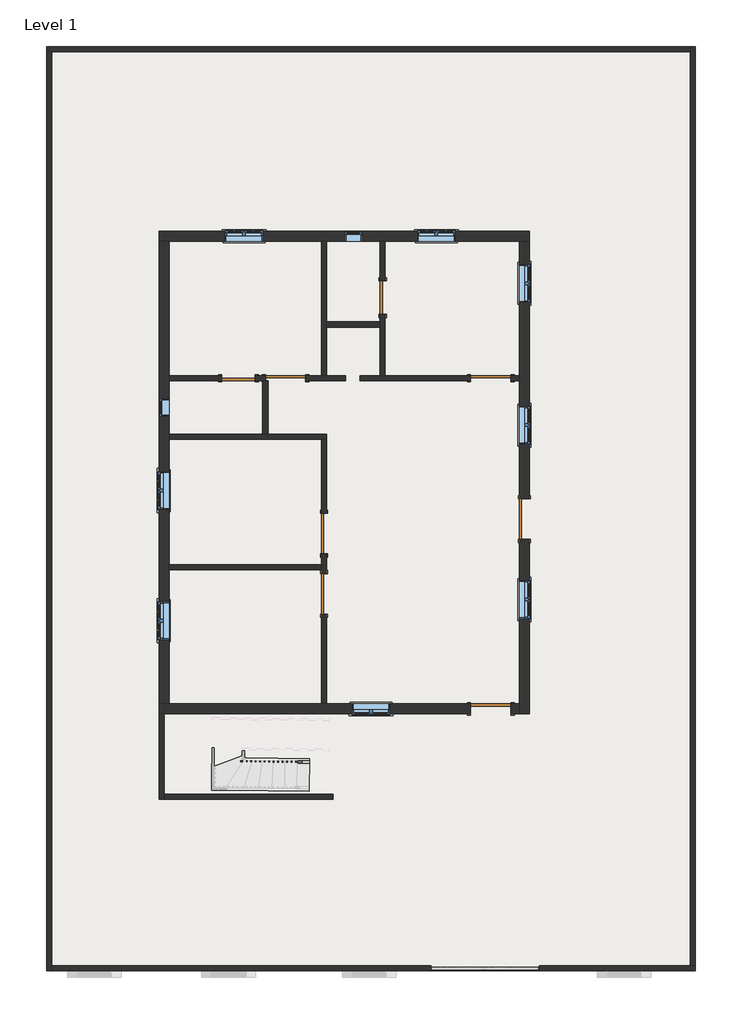
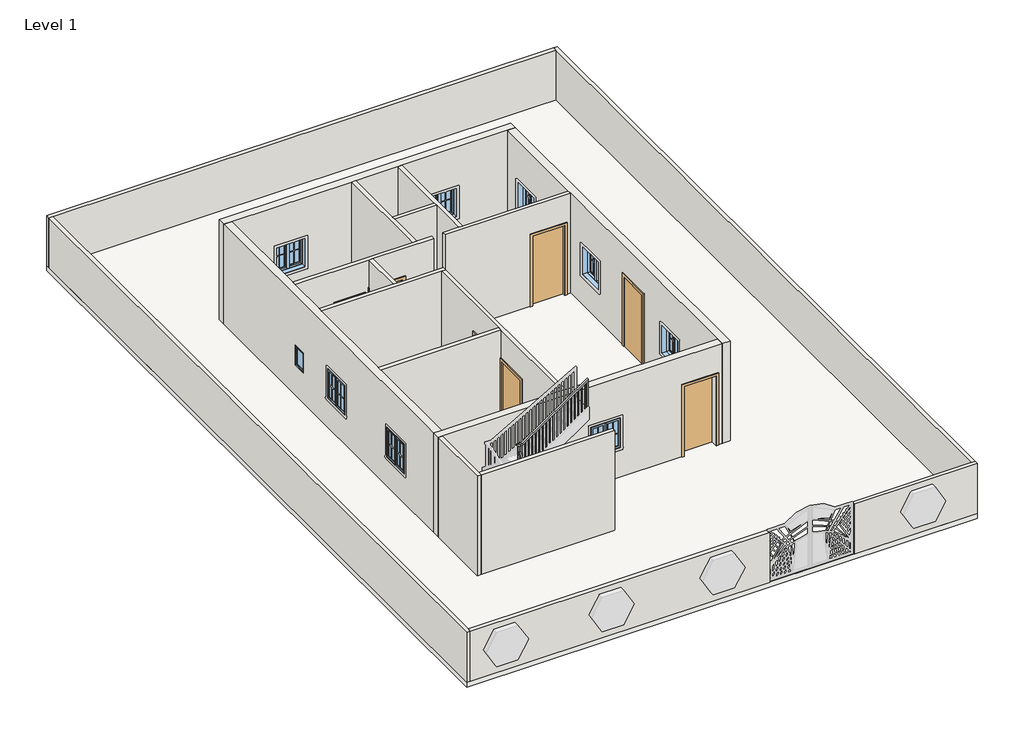
# One storey, part 1 of 2: 20 walls, 10 windows, 8 doors, 1 railing, 1 slab.
"""IFC4 building model written with IfcOpenShell, lengths in millimetres."""

from ifc_helpers import new_model, si_unit, frame, origin, origin_with_axes, place, context, project, spatial, polyline, outline, extrude, faceted_brep, transform, mapped, element, save
from components import door_f2b275c1, door_e5f9f3c4, door_305aa2a5, door_a90ba1ad, door_0ca8825f, window_aa618e30, window_339605e1

model = new_model("IFC4")

# Units and contexts
model_context = context("Model", 3, world=origin())
ifc_project = project(units=[si_unit("LENGTHUNIT", "METRE", prefix="MILLI")], contexts=[model_context])

# Site, building, storey
site = spatial("IfcSite", under=ifc_project)
building = spatial("IfcBuilding", under=site)
storey = spatial("IfcBuildingStorey", under=building, Name="Level 1", Elevation=0.0)

# Doors
placement = place(None, origin())
door_shape = door_f2b275c1(model_context)
element("IfcDoor", 1, ObjectType="Single-Flush : 30\" x 80\"", at=placement, inside=storey, context=model_context, shape_type="MappedRepresentation", body=[
    mapped(door_shape, transform((-295.4747832, 5557.2532079, 0.0), x_axis=(0.0, -1.0, 0.0), y_axis=(1.0, 0.0, 0.0), z_axis=(0.0, 0.0, 1.0))),
])
element("IfcDoor", 2, ObjectType="Single-Flush : 30\" x 80\"", at=placement, inside=storey, context=model_context, shape_type="MappedRepresentation", body=[
    mapped(door_shape, transform((-3572.0747832, 3728.4532079, 0.0), x_axis=(1.0, 0.0, 0.0), y_axis=(0.0, 1.0, 0.0), z_axis=(0.0, 0.0, 1.0))),
])
door_2_shape = door_e5f9f3c4(model_context)
element("IfcDoor", 3, ObjectType="Single-Flush : 36\" x 84\"", at=placement, inside=storey, context=model_context, shape_type="MappedRepresentation", body=[
    mapped(door_2_shape, transform((-2505.2747832, 3728.4532079, 0.0), x_axis=(1.0, 0.0, 0.0), y_axis=(0.0, 1.0, 0.0), z_axis=(0.0, 0.0, 1.0))),
])
element("IfcDoor", 4, ObjectType="Single-Flush : 36\" x 84\"", at=placement, inside=storey, context=model_context, shape_type="MappedRepresentation", body=[
    mapped(door_2_shape, transform((2161.9752168, 3728.4532079, 0.0), x_axis=(1.0, 0.0, 0.0), y_axis=(0.0, 1.0, 0.0), z_axis=(0.0, 0.0, 1.0))),
])
element("IfcDoor", 5, ObjectType="Single-Flush : 36\" x 84\"", at=placement, inside=storey, context=model_context, shape_type="MappedRepresentation", body=[
    mapped(door_2_shape, transform((-1628.9747832, -1173.7467921, 0.0), x_axis=(0.0, 1.0, 0.0), y_axis=(-1.0, 0.0, 0.0), z_axis=(0.0, 0.0, 1.0))),
])
door_3_shape = door_305aa2a5(model_context)
element("IfcDoor", 6, ObjectType="Single-Flush : 36\" x 84\"", at=placement, inside=storey, context=model_context, shape_type="MappedRepresentation", body=[
    mapped(door_3_shape, transform((-1628.9747832, 197.8532079, 0.0), x_axis=(0.0, -1.0, 0.0), y_axis=(1.0, 0.0, 0.0), z_axis=(0.0, 0.0, 1.0))),
])
door_4_shape = door_a90ba1ad(model_context)
element("IfcDoor", 7, ObjectType="Single-Flush : 36\" x 84\"", at=placement, inside=storey, context=model_context, shape_type="MappedRepresentation", body=[
    mapped(door_4_shape, transform((2923.9752168, 528.0532079, 0.0), x_axis=(0.0, -1.0, 0.0), y_axis=(1.0, 0.0, 0.0), z_axis=(0.0, 0.0, 1.0))),
])
door_5_shape = door_0ca8825f(model_context)
element("IfcDoor", 8, ObjectType="Single-Flush : 36\" x 84\"", at=placement, inside=storey, context=model_context, shape_type="MappedRepresentation", body=[
    mapped(door_5_shape, transform((2161.9752168, -3783.5967921, 0.0), x_axis=(1.0, 0.0, 0.0), y_axis=(0.0, 1.0, 0.0), z_axis=(0.0, 0.0, 1.0))),
])

# Railing
element("IfcRailing", 9, ObjectType="Handrail - Rectangular", at=placement, inside=storey, context=model_context, shape_type="SolidModel", body=[
    faceted_brep([(-1962.1803506, -5016.2038017, 1083.7333333), (-1962.1803506, -5016.2038017, 1022.2793596), (-1961.6349602, -4965.4067295, 1022.2793596), (-1961.6349602, -4965.4067295, 1083.7333333), (-3413.6283866, -5000.6201116, 2071.8756169), (-3464.4254588, -5000.0747212, 2045.0041661), (-3463.8800684, -4949.2776489, 2045.0041661), (-3413.0829962, -4949.8230393, 2071.8756169), (-3413.6283866, -5000.6201116, 2288.961538), (-3464.4254588, -5000.0747212, 2238.161538), (-3463.8800684, -4949.2776489, 2238.161538), (-3413.0829962, -4949.8230393, 2288.961538), (-3540.6210672, -4999.2566356, 2288.961538), (-3540.6210672, -4999.2566356, 2238.161538), (-3489.2786045, -4949.0049537, 2238.161538), (-3489.2786045, -4949.0049537, 2288.961538), (-3539.2575912, -4872.2639549, 2288.961538), (-3538.9677931, -4845.272478, 2238.161538), (-3488.1707209, -4845.8178684, 2238.161538), (-3488.4605189, -4872.8093453, 2288.961538), (-3537.8941152, -4745.2712743, 2477.0249579), (-3537.3487248, -4694.4742021, 2461.4786564), (-3486.5516525, -4695.0195925, 2461.4786564), (-3487.0970429, -4745.8166647, 2477.0249579), (-3537.8941152, -4745.2712743, 2645.076961), (-3537.3487248, -4694.4742021, 2594.276961), (-3486.5516525, -4695.0195925, 2594.276961), (-3487.0970429, -4745.8166647, 2645.076961), (-3536.5306392, -4618.2785937, 2645.076961), (-3536.5306392, -4618.2785937, 2594.276961), (-3486.2789573, -4669.6210563, 2594.276961), (-3486.2789573, -4669.6210563, 2645.076961), (-3409.5379585, -4619.6420697, 2645.076961), (-3393.6525863, -4619.8126254, 2594.276961), (-3394.1979767, -4670.6096976, 2594.276961), (-3410.0833489, -4670.439142, 2645.076961), (-1509.4062983, -4640.0431191, 3962.4), (-1509.9516887, -4690.8401913, 3962.4), (-1509.9516887, -4690.8401913, 3900.5869912), (-1509.4062983, -4640.0431191, 3900.5869912)], [[[0, 1, 2, 3]], [[1, 0, 4, 5]], [[2, 1, 5, 6]], [[3, 2, 6, 7]], [[0, 3, 7, 4]], [[5, 4, 8, 9]], [[6, 5, 9, 10]], [[7, 6, 10, 11]], [[4, 7, 11, 8]], [[9, 8, 12, 13]], [[10, 9, 13, 14]], [[11, 10, 14, 15]], [[8, 11, 15, 12]], [[13, 12, 16, 17]], [[14, 13, 17, 18]], [[15, 14, 18, 19]], [[12, 15, 19, 16]], [[17, 16, 20, 21]], [[18, 17, 21, 22]], [[19, 18, 22, 23]], [[16, 19, 23, 20]], [[21, 20, 24, 25]], [[22, 21, 25, 26]], [[23, 22, 26, 27]], [[20, 23, 27, 24]], [[25, 24, 28, 29]], [[26, 25, 29, 30]], [[27, 26, 30, 31]], [[24, 27, 31, 28]], [[29, 28, 32, 33]], [[30, 29, 33, 34]], [[31, 30, 34, 35]], [[28, 31, 35, 32]], [[36, 37, 38, 39]], [[33, 32, 36, 39]], [[34, 33, 39, 38]], [[35, 34, 38, 37]], [[32, 35, 37, 36]]]),
    extrude(outline(polyline([(221.9968897, -19.05), (235.2031102, 0.0), (1200.994449, 0.0), (1200.994449, -19.05), (221.9968897, -19.05)])), frame((-1590.7427644, -4674.0968508, 4079.6611157), z_axis=(0.01073603161956521, 0.9999423671517594, 0.0), x_axis=(0.0, 0.0, -1.0)), (0.0, 0.0, 1.0), 19.05),
    extrude(outline(polyline([(221.9968898, -19.05), (235.2031102, 0.0), (1130.5612733, 0.0), (1130.5612733, -19.05), (221.9968898, -19.05)])), frame((-1692.3369089, -4673.00607, 4009.22794), z_axis=(0.01073603161956521, 0.9999423671517594, 0.0), x_axis=(0.0, 0.0, -1.0)), (0.0, 0.0, 1.0), 19.05),
    extrude(outline(polyline([(221.9968897, -19.05), (235.2031102, 0.0), (1060.1280975, 0.0), (1060.1280975, -19.05), (221.9968897, -19.05)])), frame((-1793.9310534, -4671.9152892, 3938.7947642), z_axis=(0.01073603161956521, 0.9999423671517594, 0.0), x_axis=(0.0, 0.0, -1.0)), (0.0, 0.0, 1.0), 19.05),
    extrude(outline(polyline([(221.9968898, -19.05), (235.2031103, 0.0), (1159.0282552, 0.0), (1159.0282552, -19.05), (221.9968898, -19.05)])), frame((-1895.5251979, -4670.8245084, 3868.3615885), z_axis=(0.01073603161956521, 0.9999423671517594, 0.0), x_axis=(0.0, 0.0, -1.0)), (0.0, 0.0, 1.0), 19.05),
    extrude(outline(polyline([(221.9968898, -19.05), (235.2031102, 0.0), (1088.5950794, 0.0), (1088.5950794, -19.05), (221.9968898, -19.05)])), frame((-1997.1193424, -4669.7337275, 3797.9284127), z_axis=(0.01073603161956521, 0.9999423671517594, 0.0), x_axis=(0.0, 0.0, -1.0)), (0.0, 0.0, 1.0), 19.05),
    extrude(outline(polyline([(221.9968898, -19.05), (235.2031103, 0.0), (1187.495237, 0.0), (1187.495237, -19.05), (221.9968898, -19.05)])), frame((-2098.7134869, -4668.6429467, 3727.495237), z_axis=(0.01073603161956521, 0.9999423671517594, 0.0), x_axis=(0.0, 0.0, -1.0)), (0.0, 0.0, 1.0), 19.05),
    extrude(outline(polyline([(221.9968898, -19.05), (235.2031102, 0.0), (1117.0620612, 0.0), (1117.0620612, -19.05), (221.9968898, -19.05)])), frame((-2200.3076314, -4667.5521659, 3657.0620612), z_axis=(0.01073603161956521, 0.9999423671517594, 0.0), x_axis=(0.0, 0.0, -1.0)), (0.0, 0.0, 1.0), 19.05),
    extrude(outline(polyline([(221.9968897, -19.0499999), (235.2031102, 0.0), (1046.6288854, 0.0), (1046.6288854, -19.0499999), (221.9968897, -19.0499999)])), frame((-2301.9017759, -4666.4613851, 3586.6288854), z_axis=(0.01073603161956521, 0.9999423671517594, 0.0), x_axis=(0.0, 0.0, -1.0)), (0.0, 0.0, 1.0), 19.05),
    extrude(outline(polyline([(221.9968898, -19.0499999), (235.2031102, 0.0), (1145.529043, 0.0), (1145.529043, -19.0499999), (221.9968898, -19.0499999)])), frame((-2403.4959204, -4665.3706043, 3516.1957097), z_axis=(0.01073603161956521, 0.9999423671517594, 0.0), x_axis=(0.0, 0.0, -1.0)), (0.0, 0.0, 1.0), 19.05),
    extrude(outline(polyline([(221.9968897, -19.05), (235.2031102, 0.0), (1075.0958672, 0.0), (1075.0958672, -19.05), (221.9968897, -19.05)])), frame((-2505.090065, -4664.2798235, 3445.7625339), z_axis=(0.01073603161956521, 0.9999423671517594, 0.0), x_axis=(0.0, 0.0, -1.0)), (0.0, 0.0, 1.0), 19.05),
    extrude(outline(polyline([(221.9968898, -19.05), (235.2031103, 0.0), (1004.6626915, 0.0), (1004.6626915, -19.05), (221.9968898, -19.05)])), frame((-2606.6842095, -4663.1890427, 3375.3293582), z_axis=(0.01073603161956521, 0.9999423671517594, 0.0), x_axis=(0.0, 0.0, -1.0)), (0.0, 0.0, 1.0), 19.05),
    extrude(outline(polyline([(221.9968898, -19.05), (235.2031102, 0.0), (1103.5628491, 0.0), (1103.5628491, -19.05), (221.9968898, -19.05)])), frame((-2708.278354, -4662.0982619, 3304.8961824), z_axis=(0.01073603161956521, 0.9999423671517594, 0.0), x_axis=(0.0, 0.0, -1.0)), (0.0, 0.0, 1.0), 19.05),
    extrude(outline(polyline([(221.9968898, -19.05), (235.2031103, 0.0), (1033.1296734, 0.0), (1033.1296734, -19.05), (221.9968898, -19.05)])), frame((-2809.8724985, -4661.007481, 3234.4630067), z_axis=(0.01073603161956521, 0.9999423671517594, 0.0), x_axis=(0.0, 0.0, -1.0)), (0.0, 0.0, 1.0), 19.05),
    extrude(outline(polyline([(221.9968898, -19.05), (235.2031102, 0.0), (1132.0298309, 0.0), (1132.0298309, -19.05), (221.9968898, -19.05)])), frame((-2911.466643, -4659.9167002, 3164.0298309), z_axis=(0.01073603161956521, 0.9999423671517594, 0.0), x_axis=(0.0, 0.0, -1.0)), (0.0, 0.0, 1.0), 19.05),
    extrude(outline(polyline([(221.9968897, -19.05), (235.2031102, 0.0), (1061.5966551, 0.0), (1061.5966551, -19.05), (221.9968897, -19.05)])), frame((-3013.0607875, -4658.8259194, 3093.5966551), z_axis=(0.01073603161956521, 0.9999423671517594, 0.0), x_axis=(0.0, 0.0, -1.0)), (0.0, 0.0, 1.0), 19.05),
    extrude(outline(polyline([(221.9968898, -19.05), (235.2031102, 0.0), (991.1634794, 0.0), (991.1634794, -19.05), (221.9968898, -19.05)])), frame((-3114.654932, -4657.7351386, 3023.1634794), z_axis=(0.01073603161956521, 0.9999423671517594, 0.0), x_axis=(0.0, 0.0, -1.0)), (0.0, 0.0, 1.0), 19.05),
    extrude(outline(polyline([(221.9968897, -19.05), (235.2031102, 0.0), (1090.0636369, 0.0), (1090.0636369, -19.05), (221.9968897, -19.05)])), frame((-3216.2490765, -4656.6443578, 2952.7303036), z_axis=(0.01073603161956521, 0.9999423671517594, 0.0), x_axis=(0.0, 0.0, -1.0)), (0.0, 0.0, 1.0), 19.05),
    extrude(outline(polyline([(221.9968898, -19.05), (235.2031103, 0.0), (1019.6304612, 0.0), (1019.6304612, -19.05), (221.9968898, -19.05)])), frame((-3317.843221, -4655.553577, 2882.2971279), z_axis=(0.01073603161956521, 0.9999423671517594, 0.0), x_axis=(0.0, 0.0, -1.0)), (0.0, 0.0, 1.0), 19.05),
    extrude(outline(polyline([(221.9968898, -19.05), (235.2031102, 0.0), (1118.5306188, 0.0), (1118.5306188, -19.05), (221.9968898, -19.05)])), frame((-3419.4373655, -4654.4627962, 2811.8639521), z_axis=(0.01073603161956521, 0.9999423671517594, 0.0), x_axis=(0.0, 0.0, -1.0)), (0.0, 0.0, 1.0), 19.05),
    extrude(outline(polyline([(-3502.2553031, -4678.9750729), (-3521.3042052, -4678.7705515), (-3521.0996838, -4659.7216494), (-3502.0507817, -4659.9261708), (-3502.2553031, -4678.9750729)])), frame((0.0, 0.0, 1524.0), z_axis=(0.0, 0.0, 1.0), x_axis=(1.0, 0.0, 0.0)), (0.0, 0.0, 1.0), 1070.276961),
    extrude(outline(polyline([(214.4952435, -19.05), (242.7047565, 0.0), (1222.5739377, 0.0), (1222.5739377, -19.05), (214.4952435, -19.05)])), frame((-3503.3460839, -4780.5692174, 2577.2406044), z_axis=(-0.9999423671517594, 0.010736031619565895, 0.0), x_axis=(0.0, 0.0, -1.0)), (0.0, 0.0, 1.0), 19.05),
    extrude(outline(polyline([(214.4952435, -19.05), (242.7047565, 0.0), (1072.1232018, 0.0), (1072.1232018, -19.05), (214.4952435, -19.05)])), frame((-3504.4368647, -4882.1633619, 2426.7898685), z_axis=(-0.9999423671517594, 0.010736031619565895, 0.0), x_axis=(0.0, 0.0, -1.0)), (0.0, 0.0, 1.0), 19.05),
    extrude(outline(polyline([(-3476.1931112, -4965.0213631), (-3476.3976326, -4984.0702652), (-3495.4465347, -4983.8657438), (-3495.2420133, -4964.8168417), (-3476.1931112, -4965.0213631)])), frame((0.0, 0.0, 1185.3333333), z_axis=(0.0, 0.0, 1.0), x_axis=(1.0, 0.0, 0.0)), (0.0, 0.0, 1.0), 1052.8282047),
    extrude(outline(polyline([(235.0842231, -19.05), (222.115777, 0.0), (1203.1900014, 0.0), (1203.1900014, -19.05), (235.0842231, -19.05)])), frame((-3393.8523902, -4984.9565246, 2219.1900014), z_axis=(0.01073603161956537, 0.9999423671517593, 0.0), x_axis=(0.0, 0.0, -1.0)), (0.0, 0.0, 1.0), 19.05),
    extrude(outline(polyline([(235.084223, -19.05), (222.1157769, 0.0), (1134.0249555, 0.0), (1134.0249555, -19.05), (235.084223, -19.05)])), frame((-3292.2582457, -4986.0473054, 2150.0249555), z_axis=(0.01073603161956537, 0.9999423671517593, 0.0), x_axis=(0.0, 0.0, -1.0)), (0.0, 0.0, 1.0), 19.05),
    extrude(outline(polyline([(235.0842231, -19.05), (222.115777, 0.0), (1234.193243, 0.0), (1234.193243, -19.05), (235.0842231, -19.05)])), frame((-3190.6641012, -4987.1380862, 2080.8599097), z_axis=(0.01073603161956537, 0.9999423671517593, 0.0), x_axis=(0.0, 0.0, -1.0)), (0.0, 0.0, 1.0), 19.05),
    extrude(outline(polyline([(235.084223, -19.05), (222.1157769, 0.0), (1165.0281971, 0.0), (1165.0281971, -19.05), (235.084223, -19.05)])), frame((-3089.0699567, -4988.228867, 2011.6948638), z_axis=(0.01073603161956537, 0.9999423671517593, 0.0), x_axis=(0.0, 0.0, -1.0)), (0.0, 0.0, 1.0), 19.05),
    extrude(outline(polyline([(235.084223, -19.05), (222.1157769, 0.0), (1265.1964847, 0.0), (1265.1964847, -19.05), (235.084223, -19.05)])), frame((-2987.4758122, -4989.3196478, 1942.529818), z_axis=(0.01073603161956537, 0.9999423671517593, 0.0), x_axis=(0.0, 0.0, -1.0)), (0.0, 0.0, 1.0), 19.05),
    extrude(outline(polyline([(235.0842231, -19.05), (222.115777, 0.0), (1196.0314389, 0.0), (1196.0314389, -19.05), (235.0842231, -19.05)])), frame((-2885.8816677, -4990.4104286, 1873.3647722), z_axis=(0.01073603161956537, 0.9999423671517593, 0.0), x_axis=(0.0, 0.0, -1.0)), (0.0, 0.0, 1.0), 19.05),
    extrude(outline(polyline([(235.084223, -19.05), (222.1157769, 0.0), (1296.1997263, 0.0), (1296.1997263, -19.05), (235.084223, -19.05)])), frame((-2784.2875232, -4991.5012094, 1804.1997263), z_axis=(0.01073603161956537, 0.9999423671517593, 0.0), x_axis=(0.0, 0.0, -1.0)), (0.0, 0.0, 1.0), 19.05),
    extrude(outline(polyline([(235.0842231, -19.05), (222.115777, 0.0), (1227.0346805, 0.0), (1227.0346805, -19.05), (235.0842231, -19.05)])), frame((-2682.6933787, -4992.5919903, 1735.0346805), z_axis=(0.01073603161956537, 0.9999423671517593, 0.0), x_axis=(0.0, 0.0, -1.0)), (0.0, 0.0, 1.0), 19.05),
    extrude(outline(polyline([(235.084223, -19.05), (222.1157769, 0.0), (1157.8696346, 0.0), (1157.8696346, -19.05), (235.084223, -19.05)])), frame((-2581.0992342, -4993.6827711, 1665.8696346), z_axis=(0.01073603161956537, 0.9999423671517593, 0.0), x_axis=(0.0, 0.0, -1.0)), (0.0, 0.0, 1.0), 19.05),
    extrude(outline(polyline([(235.0842231, -19.05), (222.115777, 0.0), (1258.0379221, 0.0), (1258.0379221, -19.05), (235.0842231, -19.05)])), frame((-2479.5050897, -4994.7735519, 1596.7045888), z_axis=(0.01073603161956537, 0.9999423671517593, 0.0), x_axis=(0.0, 0.0, -1.0)), (0.0, 0.0, 1.0), 19.05),
    extrude(outline(polyline([(235.084223, -19.05), (222.1157769, 0.0), (1188.8728762, 0.0), (1188.8728762, -19.05), (235.084223, -19.05)])), frame((-2377.9109452, -4995.8643327, 1527.5395429), z_axis=(0.01073603161956537, 0.9999423671517593, 0.0), x_axis=(0.0, 0.0, -1.0)), (0.0, 0.0, 1.0), 19.05),
    extrude(outline(polyline([(235.084223, -19.05), (222.115777, 0.0), (1119.7078304, 0.0), (1119.7078304, -19.05), (235.084223, -19.05)])), frame((-2276.3168007, -4996.9551135, 1458.3744971), z_axis=(0.01073603161956537, 0.9999423671517593, 0.0), x_axis=(0.0, 0.0, -1.0)), (0.0, 0.0, 1.0), 19.05),
    extrude(outline(polyline([(235.0842231, -19.05), (222.115777, 0.0), (1219.876118, 0.0), (1219.876118, -19.05), (235.0842231, -19.05)])), frame((-2174.7226562, -4998.0458943, 1389.2094513), z_axis=(0.01073603161956537, 0.9999423671517593, 0.0), x_axis=(0.0, 0.0, -1.0)), (0.0, 0.0, 1.0), 19.05),
    extrude(outline(polyline([(235.084223, -19.05), (222.1157769, 0.0), (1150.7110721, 0.0), (1150.7110721, -19.05), (235.084223, -19.05)])), frame((-2073.1285117, -4999.1366751, 1320.0444054), z_axis=(0.01073603161956537, 0.9999423671517593, 0.0), x_axis=(0.0, 0.0, -1.0)), (0.0, 0.0, 1.0), 19.05),
    extrude(outline(polyline([(-3501.9826079, -4653.5765368), (-3521.03151, -4653.3720154), (-3520.8269886, -4634.3231133), (-3501.7780865, -4634.5276347), (-3501.9826079, -4653.5765368)])), frame((0.0, 0.0, 1524.0), z_axis=(0.0, 0.0, 1.0), x_axis=(1.0, 0.0, 0.0)), (0.0, 0.0, 1.0), 1070.276961),
    extrude(outline(polyline([(-3505.3231241, -4964.7086043), (-3505.5276455, -4983.7575064), (-3524.5765476, -4983.552985), (-3524.3720262, -4964.5040829), (-3505.3231241, -4964.7086043)])), frame((0.0, 0.0, 1185.3333333), z_axis=(0.0, 0.0, 1.0), x_axis=(1.0, 0.0, 0.0)), (0.0, 0.0, 1.0), 1052.8282047),
    extrude(outline(polyline([(221.9968897, -19.05), (235.2031102, 0.0), (1243.9172142, 0.0), (1243.9172142, -19.05), (221.9968897, -19.05)])), frame((-1528.8301563, -4674.7615848, 4122.5838809), z_axis=(0.01073603161956521, 0.9999423671517594, 0.0), x_axis=(0.0, 0.0, -1.0)), (0.0, 0.0, 1.0), 19.05),
    extrude(outline(polyline([(235.084223, -19.05), (222.1157769, 0.0), (1088.0302493, 0.0), (1088.0302493, -19.05), (235.084223, -19.05)])), frame((-1981.0588182, -5000.1251952, 1257.3635826), z_axis=(0.01073603161956537, 0.9999423671517593, 0.0), x_axis=(0.0, 0.0, -1.0)), (0.0, 0.0, 1.0), 19.05),
])

# Slab
element("IfcSlab", 10, ObjectType="Generic - 12\"", at=placement, inside=storey, context=model_context, shape_type="SweptSolid", body=[
    extrude(outline(polyline([(6808.4593371, 11261.08634), (6808.4593371, -9732.01366), (-7936.2406629, -9732.01366), (-7936.2406629, 11261.08634), (6808.4593371, 11261.08634)])), frame((0.0, 0.0, -152.4), z_axis=(0.0, 0.0, 1.0), x_axis=(1.0, 0.0, 0.0)), (0.0, 0.0, 1.0), 152.4),
])

# Walls
element("IfcWall", 11, ObjectType="WALL4.5\"", at=placement, inside=storey, context=model_context, shape_type="Brep", body=[
    faceted_brep([(-2048.0747832, 3671.3032079, 2133.6), (-2048.0747832, 3671.3032079, 0.0), (-1141.0287494, 3671.3032079, 0.0), (-1141.0287494, 3671.3032079, 3048.0), (-2905.3247832, 3671.3032079, 3048.0), (-3019.6247832, 3671.3032079, 3048.0), (-5153.2247832, 3671.3032079, 3048.0), (-5153.2247832, 3671.3032079, 0.0), (-3953.0747832, 3671.3032079, 0.0), (-3953.0747832, 3671.3032079, 2032.0), (-3191.0747832, 3671.3032079, 2032.0), (-3191.0747832, 3671.3032079, 0.0), (-3019.6247832, 3671.3032079, 0.0), (-2962.4747832, 3671.3032079, 0.0), (-2962.4747832, 3671.3032079, 2133.6), (-1141.0287494, 3785.6032079, 0.0), (-1571.8247832, 3785.6032079, 0.0), (-1686.1247832, 3785.6032079, 0.0), (-2048.0747832, 3785.6032079, 0.0), (-2048.0747832, 3785.6032079, 2133.6), (-2962.4747832, 3785.6032079, 2133.6), (-2962.4747832, 3785.6032079, 0.0), (-3191.0747832, 3785.6032079, 0.0), (-3191.0747832, 3785.6032079, 2032.0), (-3953.0747832, 3785.6032079, 2032.0), (-3953.0747832, 3785.6032079, 0.0), (-5153.2247832, 3785.6032079, 0.0), (-5153.2247832, 3785.6032079, 3048.0), (-1686.1247832, 3785.6032079, 3048.0), (-1571.8247832, 3785.6032079, 3048.0), (-1141.0287494, 3785.6032079, 3048.0)], [[[0, 1, 2, 3, 4, 5, 6, 7, 8, 9, 10, 11, 12, 13, 14]], [[15, 16, 17, 18, 19, 20, 21, 22, 23, 24, 25, 26, 27, 28, 29, 30]], [[8, 7, 26, 25]], [[2, 1, 18, 17, 16, 15]], [[13, 12, 11, 22, 21]], [[3, 2, 15, 30]], [[7, 6, 27, 26]], [[23, 22, 11, 10]], [[24, 23, 10, 9]], [[25, 24, 9, 8]], [[19, 18, 1, 0]], [[20, 19, 0, 14]], [[21, 20, 14, 13]], [[6, 5, 4, 3, 30, 29, 28, 27]]]),
])
element("IfcWall", 12, ObjectType="WALL4.5\"", at=placement, inside=storey, context=model_context, shape_type="Brep", body=[
    faceted_brep([(2619.1752168, 3671.3032079, 2133.6), (2619.1752168, 3671.3032079, 0.0), (2809.6752168, 3671.3032079, 0.0), (2809.6752168, 3671.3032079, 3048.0), (-812.7163761, 3671.3032079, 3048.0), (-812.7163761, 3671.3032079, 0.0), (1704.7752168, 3671.3032079, 0.0), (1704.7752168, 3671.3032079, 2133.6), (2809.6752168, 3785.6032079, 0.0), (2619.1752168, 3785.6032079, 0.0), (2619.1752168, 3785.6032079, 2133.6), (1704.7752168, 3785.6032079, 2133.6), (1704.7752168, 3785.6032079, 0.0), (-238.3247832, 3785.6032079, 0.0), (-352.6247832, 3785.6032079, 0.0), (-812.7163761, 3785.6032079, 0.0), (-812.7163761, 3785.6032079, 3048.0), (-352.6247832, 3785.6032079, 3048.0), (-238.3247832, 3785.6032079, 3048.0), (2809.6752168, 3785.6032079, 3048.0)], [[[0, 1, 2, 3, 4, 5, 6, 7]], [[8, 9, 10, 11, 12, 13, 14, 15, 16, 17, 18, 19]], [[6, 5, 15, 14, 13, 12]], [[2, 1, 9, 8]], [[5, 4, 16, 15]], [[3, 2, 8, 19]], [[10, 9, 1, 0]], [[11, 10, 0, 7]], [[12, 11, 7, 6]], [[4, 3, 19, 18, 17, 16]]]),
])
element("IfcWall", 13, ObjectType="WALL4.5\"", at=placement, inside=storey, context=model_context, shape_type="Brep", body=[
    faceted_brep([(-1686.1247832, 6833.6032079, 0.0), (-1686.1247832, 3785.6032079, 0.0), (-1686.1247832, 3785.6032079, 3048.0), (-1686.1247832, 6833.6032079, 3048.0), (-1571.8247832, 6833.6032079, 0.0), (-1571.8247832, 6833.6032079, 3048.0), (-1571.8247832, 5004.8032079, 3048.0), (-1571.8247832, 4890.5032079, 3048.0), (-1571.8247832, 3785.6032079, 3048.0), (-1571.8247832, 3785.6032079, 0.0), (-1571.8247832, 4890.5032079, 0.0), (-1571.8247832, 5004.8032079, 0.0)], [[[0, 1, 2, 3]], [[4, 5, 6, 7, 8, 9, 10, 11]], [[1, 0, 4, 11, 10, 9]], [[0, 3, 5, 4]], [[2, 1, 9, 8]], [[3, 2, 8, 7, 6, 5]]]),
])
element("IfcWall", 14, ObjectType="WALL4.5\"", at=placement, inside=storey, context=model_context, shape_type="SweptSolid", body=[
    extrude(outline(polyline([(-352.6247832, 4890.5032079), (-1571.8247832, 4890.5032079), (-1571.8247832, 5004.8032079), (-352.6247832, 5004.8032079), (-352.6247832, 4890.5032079)])), origin_with_axes(), (0.0, 0.0, 1.0), 3048.0),
])
element("IfcWall", 15, ObjectType="WALL4.5\"", at=placement, inside=storey, context=model_context, shape_type="Brep", body=[
    faceted_brep([(-352.6247832, 5176.2532079, 2032.0), (-352.6247832, 5176.2532079, 0.0), (-352.6247832, 5004.8032079, 0.0), (-352.6247832, 4890.5032079, 0.0), (-352.6247832, 3785.6032079, 0.0), (-352.6247832, 3785.6032079, 3048.0), (-352.6247832, 4890.5032079, 3048.0), (-352.6247832, 5004.8032079, 3048.0), (-352.6247832, 6833.6032079, 3048.0), (-352.6247832, 6833.6032079, 0.0), (-352.6247832, 5938.2532079, 0.0), (-352.6247832, 5938.2532079, 2032.0), (-238.3247832, 3785.6032079, 0.0), (-238.3247832, 5176.2532079, 0.0), (-238.3247832, 5176.2532079, 2032.0), (-238.3247832, 5938.2532079, 2032.0), (-238.3247832, 5938.2532079, 0.0), (-238.3247832, 6833.6032079, 0.0), (-238.3247832, 6833.6032079, 3048.0), (-238.3247832, 3785.6032079, 3048.0)], [[[0, 1, 2, 3, 4, 5, 6, 7, 8, 9, 10, 11]], [[12, 13, 14, 15, 16, 17, 18, 19]], [[10, 9, 17, 16]], [[4, 3, 2, 1, 13, 12]], [[9, 8, 18, 17]], [[5, 4, 12, 19]], [[14, 13, 1, 0]], [[15, 14, 0, 11]], [[16, 15, 11, 10]], [[8, 7, 6, 5, 19, 18]]]),
])
element("IfcWall", 16, ObjectType="WALL4.5\"", at=placement, inside=storey, context=model_context, shape_type="Brep", body=[
    faceted_brep([(-3019.6247832, 3671.3032079, 0.0), (-3019.6247832, 2452.1032079, 0.0), (-3019.6247832, 2452.1032079, 3048.0), (-3019.6247832, 3671.3032079, 3048.0), (-2905.3247832, 3671.3032079, 0.0), (-2905.3247832, 3671.3032079, 3048.0), (-2905.3247832, 2452.1032079, 3048.0), (-2905.3247832, 2452.1032079, 0.0), (-2962.4747832, 3671.3032079, 0.0)], [[[0, 1, 2, 3]], [[4, 5, 6, 7]], [[1, 0, 8, 4, 7]], [[0, 3, 5, 4, 8]], [[2, 1, 7, 6]], [[3, 2, 6, 5]]]),
])
element("IfcWall", 17, ObjectType="WALL4.5\"", at=placement, inside=storey, context=model_context, shape_type="Brep", body=[
    faceted_brep([(-5153.2247832, 2337.8032079, 0.0), (-1686.1247832, 2337.8032079, 0.0), (-1571.8247832, 2337.8032079, 0.0), (-1571.8247832, 2337.8032079, 3048.0), (-1686.1247832, 2337.8032079, 3048.0), (-5153.2247832, 2337.8032079, 3048.0), (-5153.2247832, 2452.1032079, 0.0), (-5153.2247832, 2452.1032079, 3048.0), (-3019.6247832, 2452.1032079, 3048.0), (-2905.3247832, 2452.1032079, 3048.0), (-1571.8247832, 2452.1032079, 3048.0), (-1571.8247832, 2452.1032079, 0.0), (-2905.3247832, 2452.1032079, 0.0), (-3019.6247832, 2452.1032079, 0.0)], [[[0, 1, 2, 3, 4, 5]], [[6, 7, 8, 9, 10, 11, 12, 13]], [[2, 1, 0, 6, 13, 12, 11]], [[0, 5, 7, 6]], [[3, 2, 11, 10]], [[5, 4, 3, 10, 9, 8, 7]]]),
])
element("IfcWall", 18, ObjectType="WALL4.5\"", at=placement, inside=storey, context=model_context, shape_type="Brep", body=[
    faceted_brep([(-1686.1247832, -259.3467921, 0.0), (-1686.1247832, -506.9967921, 0.0), (-1686.1247832, -621.2967921, 0.0), (-1686.1247832, -716.5467921, 0.0), (-1686.1247832, -716.5467921, 2133.6), (-1686.1247832, -1630.9467921, 2133.6), (-1686.1247832, -1630.9467921, 0.0), (-1686.1247832, -3669.2967921, 0.0), (-1686.1247832, -3669.2967921, 3048.0), (-1686.1247832, -621.2967921, 3048.0), (-1686.1247832, -506.9967921, 3048.0), (-1686.1247832, 2337.8032079, 3048.0), (-1686.1247832, 2337.8032079, 0.0), (-1686.1247832, 655.0532079, 0.0), (-1686.1247832, 655.0532079, 2133.6), (-1686.1247832, -259.3467921, 2133.6), (-1571.8247832, -716.5467921, 2133.6), (-1571.8247832, -716.5467921, 0.0), (-1571.8247832, -259.3467921, 0.0), (-1571.8247832, -259.3467921, 2133.6), (-1571.8247832, 655.0532079, 2133.6), (-1571.8247832, 655.0532079, 0.0), (-1571.8247832, 2337.8032079, 0.0), (-1571.8247832, 2337.8032079, 3048.0), (-1571.8247832, -3669.2967921, 3048.0), (-1571.8247832, -3669.2967921, 0.0), (-1571.8247832, -1630.9467921, 0.0), (-1571.8247832, -1630.9467921, 2133.6)], [[[0, 1, 2, 3, 4, 5, 6, 7, 8, 9, 10, 11, 12, 13, 14, 15]], [[16, 17, 18, 19, 20, 21, 22, 23, 24, 25, 26, 27]], [[13, 12, 22, 21]], [[26, 25, 7, 6]], [[18, 17, 3, 2, 1, 0]], [[12, 11, 23, 22]], [[8, 7, 25, 24]], [[19, 18, 0, 15]], [[20, 19, 15, 14]], [[21, 20, 14, 13]], [[4, 3, 17, 16]], [[5, 4, 16, 27]], [[6, 5, 27, 26]], [[11, 10, 9, 8, 24, 23]]]),
])
element("IfcWall", 19, ObjectType="WALL4.5\"", at=placement, inside=storey, context=model_context, shape_type="SweptSolid", body=[
    extrude(outline(polyline([(-1686.1247832, -621.2967921), (-5153.2247832, -621.2967921), (-5153.2247832, -506.9967921), (-1686.1247832, -506.9967921), (-1686.1247832, -621.2967921)])), origin_with_axes(), (0.0, 0.0, 1.0), 3048.0),
])
element("IfcWall", 20, ObjectType="WALL4.5\"", at=placement, inside=storey, context=model_context, shape_type="Brep", body=[
    faceted_brep([(-5381.8247832, -3897.8967921, 0.0), (-5381.8247832, -5840.9967921, 0.0), (-5381.8247832, -5840.9967921, 3048.0), (-5381.8247832, -3897.8967921, 3048.0), (-5267.5247832, -3897.8967921, 0.0), (-5267.5247832, -3897.8967921, 3048.0), (-5267.5247832, -5726.6967921, 3048.0), (-5267.5247832, -5840.9967921, 3048.0), (-5267.5247832, -5840.9967921, 0.0), (-5267.5247832, -5726.6967921, 0.0)], [[[0, 1, 2, 3]], [[4, 5, 6, 7, 8, 9]], [[1, 0, 4, 9, 8]], [[0, 3, 5, 4]], [[2, 1, 8, 7]], [[3, 2, 7, 6, 5]]]),
])
element("IfcWall", 21, ObjectType="WALL4.5\"", at=placement, inside=storey, context=model_context, shape_type="SweptSolid", body=[
    extrude(outline(polyline([(-1419.4247832, -5840.9967921), (-5267.5247832, -5840.9967921), (-5267.5247832, -5726.6967921), (-1419.4247832, -5726.6967921), (-1419.4247832, -5840.9967921)])), origin_with_axes(), (0.0, 0.0, 1.0), 3048.0),
])
element("IfcWall", 22, ObjectType="WALL4.5\"", at=placement, inside=storey, context=model_context, shape_type="Brep", body=[
    faceted_brep([(-7936.2406629, 11146.78634, 0.0), (-7821.9406629, 11146.78634, 0.0), (6694.1593371, 11146.78634, 0.0), (6694.1593371, 11146.78634, 1524.0), (-7821.9406629, 11146.78634, 1524.0), (-7936.2406629, 11146.78634, 1524.0), (-7936.2406629, 11261.08634, 0.0), (-7936.2406629, 11261.08634, 1524.0), (6694.1593371, 11261.08634, 1524.0), (6694.1593371, 11261.08634, 0.0)], [[[0, 1, 2, 3, 4, 5]], [[6, 7, 8, 9]], [[2, 1, 0, 6, 9]], [[5, 4, 3, 8, 7]], [[0, 5, 7, 6]], [[3, 2, 9, 8]]]),
])
element("IfcWall", 23, ObjectType="WALL4.5\"", at=placement, inside=storey, context=model_context, shape_type="Brep", body=[
    faceted_brep([(-7821.9406629, -9732.01366, 0.0), (-7821.9406629, -9617.71366, 0.0), (-7821.9406629, 11146.78634, 0.0), (-7821.9406629, 11146.78634, 1524.0), (-7821.9406629, -9617.71366, 1524.0), (-7821.9406629, -9732.01366, 1524.0), (-7936.2406629, -9732.01366, 0.0), (-7936.2406629, -9732.01366, 1524.0), (-7936.2406629, 11146.78634, 1524.0), (-7936.2406629, 11146.78634, 0.0)], [[[0, 1, 2, 3, 4, 5]], [[6, 7, 8, 9]], [[2, 1, 0, 6, 9]], [[5, 4, 3, 8, 7]], [[0, 5, 7, 6]], [[3, 2, 9, 8]]]),
])
element("IfcWall", 24, ObjectType="WALL4.5\"", at=placement, inside=storey, context=model_context, shape_type="Brep", body=[
    faceted_brep([(6808.4593371, -9617.71366, 0.0), (6694.1593371, -9617.71366, 0.0), (3271.5093371, -9617.71366, 0.0), (3271.5093371, -9617.71366, 1524.0), (6694.1593371, -9617.71366, 1524.0), (6808.4593371, -9617.71366, 1524.0), (6808.4593371, -9732.01366, 0.0), (6808.4593371, -9732.01366, 1524.0), (3271.5093371, -9732.01366, 1524.0), (3271.5093371, -9732.01366, 0.0)], [[[0, 1, 2, 3, 4, 5]], [[6, 7, 8, 9]], [[2, 1, 0, 6, 9]], [[3, 2, 9, 8]], [[5, 4, 3, 8, 7]], [[0, 5, 7, 6]]]),
])
element("IfcWall", 25, ObjectType="WALL4.5\"", at=placement, inside=storey, context=model_context, shape_type="Brep", body=[
    faceted_brep([(6694.1593371, 11261.08634, 0.0), (6694.1593371, 11146.78634, 0.0), (6694.1593371, -9617.71366, 0.0), (6694.1593371, -9617.71366, 1524.0), (6694.1593371, 11146.78634, 1524.0), (6694.1593371, 11261.08634, 1524.0), (6808.4593371, 11261.08634, 0.0), (6808.4593371, 11261.08634, 1524.0), (6808.4593371, -9617.71366, 1524.0), (6808.4593371, -9617.71366, 0.0)], [[[0, 1, 2, 3, 4, 5]], [[6, 7, 8, 9]], [[2, 1, 0, 6, 9]], [[5, 4, 3, 8, 7]], [[0, 5, 7, 6]], [[3, 2, 9, 8]]]),
])
element("IfcWall", 26, ObjectType="WALL4.5\"", at=placement, inside=storey, context=model_context, shape_type="SweptSolid", body=[
    extrude(outline(polyline([(-7821.9406629, -9617.71366), (807.7093371, -9617.71366), (807.7093371, -9732.01366), (-7821.9406629, -9732.01366), (-7821.9406629, -9617.71366)])), origin_with_axes(), (0.0, 0.0, 1.0), 1524.0),
])
element("IfcWall", 27, ObjectType="WALL9\"", at=placement, inside=storey, context=model_context, shape_type="Brep", body=[
    faceted_brep([(-5381.8247832, 6833.6032079, 0.0), (-5153.2247832, 6833.6032079, 0.0), (-1686.1247832, 6833.6032079, 0.0), (-1571.8247832, 6833.6032079, 0.0), (-352.6247832, 6833.6032079, 0.0), (-238.3247832, 6833.6032079, 0.0), (2809.6752168, 6833.6032079, 0.0), (3038.2752168, 6833.6032079, 0.0), (3038.2752168, 6833.6032079, 3048.0), (2809.6752168, 6833.6032079, 3048.0), (-238.3247832, 6833.6032079, 3048.0), (-352.6247832, 6833.6032079, 3048.0), (-1571.8247832, 6833.6032079, 3048.0), (-1686.1247832, 6833.6032079, 3048.0), (-5153.2247832, 6833.6032079, 3048.0), (-5381.8247832, 6833.6032079, 3048.0), (-759.0247832, 6833.6032079, 1524.0), (-759.0247832, 6833.6032079, 914.4), (-1165.4247832, 6833.6032079, 914.4), (-1165.4247832, 6833.6032079, 1524.0), (-3016.4497832, 6833.6032079, 1828.8), (-3016.4497832, 6833.6032079, 914.4), (-3880.0497832, 6833.6032079, 914.4), (-3880.0497832, 6833.6032079, 1828.8), (1355.5252168, 6833.6032079, 1828.8), (1355.5252168, 6833.6032079, 914.4), (491.9252168, 6833.6032079, 914.4), (491.9252168, 6833.6032079, 1828.8), (-5381.8247832, 7062.2032079, 0.0), (-5381.8247832, 7062.2032079, 3048.0), (3038.2752168, 7062.2032079, 3048.0), (3038.2752168, 7062.2032079, 0.0), (-759.0247832, 7062.2032079, 1524.0), (-1165.4247832, 7062.2032079, 1524.0), (-1165.4247832, 7062.2032079, 914.4), (-759.0247832, 7062.2032079, 914.4), (-3016.4497832, 7062.2032079, 1828.8), (-3880.0497832, 7062.2032079, 1828.8), (-3880.0497832, 7062.2032079, 914.4), (-3016.4497832, 7062.2032079, 914.4), (1355.5252168, 7062.2032079, 1828.8), (491.9252168, 7062.2032079, 1828.8), (491.9252168, 7062.2032079, 914.4), (1355.5252168, 7062.2032079, 914.4)], [[[0, 1, 2, 3, 4, 5, 6, 7, 8, 9, 10, 11, 12, 13, 14, 15], [16, 17, 18, 19], [20, 21, 22, 23], [24, 25, 26, 27]], [[28, 29, 30, 31], [32, 33, 34, 35], [36, 37, 38, 39], [40, 41, 42, 43]], [[7, 6, 5, 4, 3, 2, 1, 0, 28, 31]], [[8, 7, 31, 30]], [[0, 15, 29, 28]], [[17, 16, 32, 35]], [[18, 17, 35, 34]], [[19, 18, 34, 33]], [[16, 19, 33, 32]], [[21, 20, 36, 39]], [[22, 21, 39, 38]], [[23, 22, 38, 37]], [[20, 23, 37, 36]], [[25, 24, 40, 43]], [[26, 25, 43, 42]], [[27, 26, 42, 41]], [[24, 27, 41, 40]], [[15, 14, 13, 12, 11, 10, 9, 8, 30, 29]]]),
])
element("IfcWall", 28, ObjectType="WALL9\"", at=placement, inside=storey, context=model_context, shape_type="Brep", body=[
    faceted_brep([(2809.6752168, 70.8532079, 2133.6), (2809.6752168, 70.8532079, 0.0), (2809.6752168, -3669.2967921, 0.0), (2809.6752168, -3897.8967921, 0.0), (2809.6752168, -3897.8967921, 3048.0), (2809.6752168, -3669.2967921, 3048.0), (2809.6752168, 3671.3032079, 3048.0), (2809.6752168, 3785.6032079, 3048.0), (2809.6752168, 6833.6032079, 3048.0), (2809.6752168, 6833.6032079, 0.0), (2809.6752168, 3785.6032079, 0.0), (2809.6752168, 3671.3032079, 0.0), (2809.6752168, 985.2532079, 0.0), (2809.6752168, 985.2532079, 2133.6), (2809.6752168, 5449.3032079, 1828.8), (2809.6752168, 5449.3032079, 914.4), (2809.6752168, 6312.9032079, 914.4), (2809.6752168, 6312.9032079, 1828.8), (2809.6752168, 2229.8532079, 1828.8), (2809.6752168, 2229.8532079, 914.4), (2809.6752168, 3093.4532079, 914.4), (2809.6752168, 3093.4532079, 1828.8), (2809.6752168, -1732.5467921, 1828.8), (2809.6752168, -1732.5467921, 914.4), (2809.6752168, -868.9467921, 914.4), (2809.6752168, -868.9467921, 1828.8), (3038.2752168, -3897.8967921, 0.0), (3038.2752168, 70.8532079, 0.0), (3038.2752168, 70.8532079, 2133.6), (3038.2752168, 985.2532079, 2133.6), (3038.2752168, 985.2532079, 0.0), (3038.2752168, 6833.6032079, 0.0), (3038.2752168, 6833.6032079, 3048.0), (3038.2752168, -3897.8967921, 3048.0), (3038.2752168, 5449.3032079, 1828.8), (3038.2752168, 6312.9032079, 1828.8), (3038.2752168, 6312.9032079, 914.4), (3038.2752168, 5449.3032079, 914.4), (3038.2752168, 2229.8532079, 1828.8), (3038.2752168, 3093.4532079, 1828.8), (3038.2752168, 3093.4532079, 914.4), (3038.2752168, 2229.8532079, 914.4), (3038.2752168, -1732.5467921, 1828.8), (3038.2752168, -868.9467921, 1828.8), (3038.2752168, -868.9467921, 914.4), (3038.2752168, -1732.5467921, 914.4)], [[[0, 1, 2, 3, 4, 5, 6, 7, 8, 9, 10, 11, 12, 13], [14, 15, 16, 17], [18, 19, 20, 21], [22, 23, 24, 25]], [[26, 27, 28, 29, 30, 31, 32, 33], [34, 35, 36, 37], [38, 39, 40, 41], [42, 43, 44, 45]], [[3, 2, 1, 27, 26]], [[12, 11, 10, 9, 31, 30]], [[9, 8, 32, 31]], [[4, 3, 26, 33]], [[28, 27, 1, 0]], [[29, 28, 0, 13]], [[30, 29, 13, 12]], [[15, 14, 34, 37]], [[16, 15, 37, 36]], [[17, 16, 36, 35]], [[14, 17, 35, 34]], [[19, 18, 38, 41]], [[20, 19, 41, 40]], [[21, 20, 40, 39]], [[18, 21, 39, 38]], [[23, 22, 42, 45]], [[24, 23, 45, 44]], [[25, 24, 44, 43]], [[22, 25, 43, 42]], [[8, 7, 6, 5, 4, 33, 32]]]),
])
element("IfcWall", 29, ObjectType="WALL9\"", at=placement, inside=storey, context=model_context, shape_type="Brep", body=[
    faceted_brep([(2809.6752168, -3669.2967921, 0.0), (2619.1752168, -3669.2967921, 0.0), (2619.1752168, -3669.2967921, 2133.6), (1704.7752168, -3669.2967921, 2133.6), (1704.7752168, -3669.2967921, 0.0), (-1571.8247832, -3669.2967921, 0.0), (-1686.1247832, -3669.2967921, 0.0), (-5153.2247832, -3669.2967921, 0.0), (-5381.8247832, -3669.2967921, 0.0), (-5381.8247832, -3669.2967921, 3048.0), (-5153.2247832, -3669.2967921, 3048.0), (-1686.1247832, -3669.2967921, 3048.0), (-1571.8247832, -3669.2967921, 3048.0), (2809.6752168, -3669.2967921, 3048.0), (-993.9747832, -3669.2967921, 1828.8), (-993.9747832, -3669.2967921, 914.4), (-130.3747832, -3669.2967921, 914.4), (-130.3747832, -3669.2967921, 1828.8), (2619.1752168, -3897.8967921, 2133.6), (2619.1752168, -3897.8967921, 0.0), (2809.6752168, -3897.8967921, 0.0), (2809.6752168, -3897.8967921, 3048.0), (-5267.5247832, -3897.8967921, 3048.0), (-5381.8247832, -3897.8967921, 3048.0), (-5381.8247832, -3897.8967921, 0.0), (-5267.5247832, -3897.8967921, 0.0), (1704.7752168, -3897.8967921, 0.0), (1704.7752168, -3897.8967921, 2133.6), (-993.9747832, -3897.8967921, 1828.8), (-130.3747832, -3897.8967921, 1828.8), (-130.3747832, -3897.8967921, 914.4), (-993.9747832, -3897.8967921, 914.4)], [[[0, 1, 2, 3, 4, 5, 6, 7, 8, 9, 10, 11, 12, 13], [14, 15, 16, 17]], [[18, 19, 20, 21, 22, 23, 24, 25, 26, 27], [28, 29, 30, 31]], [[20, 19, 1, 0]], [[26, 25, 24, 8, 7, 6, 5, 4]], [[0, 13, 21, 20]], [[9, 8, 24, 23]], [[2, 1, 19, 18]], [[3, 2, 18, 27]], [[4, 3, 27, 26]], [[15, 14, 28, 31]], [[16, 15, 31, 30]], [[17, 16, 30, 29]], [[14, 17, 29, 28]], [[13, 12, 11, 10, 9, 23, 22, 21]]]),
])
element("IfcWall", 30, ObjectType="WALL9\"", at=placement, inside=storey, context=model_context, shape_type="Brep", body=[
    faceted_brep([(-5153.2247832, -3669.2967921, 0.0), (-5153.2247832, -621.2967921, 0.0), (-5153.2247832, -506.9967921, 0.0), (-5153.2247832, 2337.8032079, 0.0), (-5153.2247832, 2452.1032079, 0.0), (-5153.2247832, 3671.3032079, 0.0), (-5153.2247832, 3785.6032079, 0.0), (-5153.2247832, 6833.6032079, 0.0), (-5153.2247832, 6833.6032079, 3048.0), (-5153.2247832, 3785.6032079, 3048.0), (-5153.2247832, 3671.3032079, 3048.0), (-5153.2247832, 2452.1032079, 3048.0), (-5153.2247832, 2337.8032079, 3048.0), (-5153.2247832, -506.9967921, 3048.0), (-5153.2247832, -621.2967921, 3048.0), (-5153.2247832, -3669.2967921, 3048.0), (-5153.2247832, 3264.9032079, 1524.0), (-5153.2247832, 3264.9032079, 914.4), (-5153.2247832, 2858.5032079, 914.4), (-5153.2247832, 2858.5032079, 1524.0), (-5153.2247832, 1607.5532079, 1828.8), (-5153.2247832, 1607.5532079, 914.4), (-5153.2247832, 743.9532079, 914.4), (-5153.2247832, 743.9532079, 1828.8), (-5153.2247832, -1351.5467921, 1828.8), (-5153.2247832, -1351.5467921, 914.4), (-5153.2247832, -2215.1467921, 914.4), (-5153.2247832, -2215.1467921, 1828.8), (-5381.8247832, -3669.2967921, 0.0), (-5381.8247832, -3669.2967921, 3048.0), (-5381.8247832, 6833.6032079, 3048.0), (-5381.8247832, 6833.6032079, 0.0), (-5381.8247832, 3264.9032079, 1524.0), (-5381.8247832, 2858.5032079, 1524.0), (-5381.8247832, 2858.5032079, 914.4), (-5381.8247832, 3264.9032079, 914.4), (-5381.8247832, 1607.5532079, 1828.8), (-5381.8247832, 743.9532079, 1828.8), (-5381.8247832, 743.9532079, 914.4), (-5381.8247832, 1607.5532079, 914.4), (-5381.8247832, -1351.5467921, 1828.8), (-5381.8247832, -2215.1467921, 1828.8), (-5381.8247832, -2215.1467921, 914.4), (-5381.8247832, -1351.5467921, 914.4)], [[[0, 1, 2, 3, 4, 5, 6, 7, 8, 9, 10, 11, 12, 13, 14, 15], [16, 17, 18, 19], [20, 21, 22, 23], [24, 25, 26, 27]], [[28, 29, 30, 31], [32, 33, 34, 35], [36, 37, 38, 39], [40, 41, 42, 43]], [[7, 6, 5, 4, 3, 2, 1, 0, 28, 31]], [[8, 7, 31, 30]], [[0, 15, 29, 28]], [[17, 16, 32, 35]], [[18, 17, 35, 34]], [[19, 18, 34, 33]], [[16, 19, 33, 32]], [[21, 20, 36, 39]], [[22, 21, 39, 38]], [[23, 22, 38, 37]], [[20, 23, 37, 36]], [[25, 24, 40, 43]], [[26, 25, 43, 42]], [[27, 26, 42, 41]], [[24, 27, 41, 40]], [[15, 14, 13, 12, 11, 10, 9, 8, 30, 29]]]),
])

# Windows
window_shape = window_aa618e30(model_context)
element("IfcWindow", 31, ObjectType="Fixed : 16\" x 24\"", at=placement, inside=storey, context=model_context, shape_type="MappedRepresentation", body=[
    mapped(window_shape, transform((-924.1247832, 6947.9032079, 0.0), x_axis=(1.0, 0.0, 0.0), y_axis=(0.0, 1.0, 0.0), z_axis=(0.0, 0.0, 1.0))),
])
element("IfcWindow", 32, ObjectType="Fixed : 16\" x 24\"", at=placement, inside=storey, context=model_context, shape_type="MappedRepresentation", body=[
    mapped(window_shape, transform((-5267.5247832, 3099.8032079, 0.0), x_axis=(0.0, 1.0, 0.0), y_axis=(-1.0, 0.0, 0.0), z_axis=(0.0, 0.0, 1.0))),
])
window_2_shape = window_339605e1(model_context)
element("IfcWindow", 33, ObjectType="Window-Casement-Double : 34\" x 36\"", at=placement, inside=storey, context=model_context, shape_type="MappedRepresentation", body=[
    mapped(window_2_shape, transform((-3448.2497832, 6947.9032079, 0.0), x_axis=(1.0, 0.0, 0.0), y_axis=(0.0, 1.0, 0.0), z_axis=(0.0, 0.0, 1.0))),
])
element("IfcWindow", 34, ObjectType="Window-Casement-Double : 34\" x 36\"", at=placement, inside=storey, context=model_context, shape_type="MappedRepresentation", body=[
    mapped(window_2_shape, transform((923.7252168, 6947.9032079, 0.0), x_axis=(1.0, 0.0, 0.0), y_axis=(0.0, 1.0, 0.0), z_axis=(0.0, 0.0, 1.0))),
])
element("IfcWindow", 35, ObjectType="Window-Casement-Double : 34\" x 36\"", at=placement, inside=storey, context=model_context, shape_type="MappedRepresentation", body=[
    mapped(window_2_shape, transform((2923.9752168, 5881.1032079, 0.0), x_axis=(0.0, -1.0, 0.0), y_axis=(1.0, 0.0, 0.0), z_axis=(0.0, 0.0, 1.0))),
])
element("IfcWindow", 36, ObjectType="Window-Casement-Double : 34\" x 36\"", at=placement, inside=storey, context=model_context, shape_type="MappedRepresentation", body=[
    mapped(window_2_shape, transform((2923.9752168, 2661.6532079, 0.0), x_axis=(0.0, -1.0, 0.0), y_axis=(1.0, 0.0, 0.0), z_axis=(0.0, 0.0, 1.0))),
])
element("IfcWindow", 37, ObjectType="Window-Casement-Double : 34\" x 36\"", at=placement, inside=storey, context=model_context, shape_type="MappedRepresentation", body=[
    mapped(window_2_shape, transform((2923.9752168, -1300.7467921, 0.0), x_axis=(0.0, -1.0, 0.0), y_axis=(1.0, 0.0, 0.0), z_axis=(0.0, 0.0, 1.0))),
])
element("IfcWindow", 38, ObjectType="Window-Casement-Double : 34\" x 36\"", at=placement, inside=storey, context=model_context, shape_type="MappedRepresentation", body=[
    mapped(window_2_shape, transform((-5267.5247832, 1175.7532079, 0.0), x_axis=(0.0, 1.0, 0.0), y_axis=(-1.0, 0.0, 0.0), z_axis=(0.0, 0.0, 1.0))),
])
element("IfcWindow", 39, ObjectType="Window-Casement-Double : 34\" x 36\"", at=placement, inside=storey, context=model_context, shape_type="MappedRepresentation", body=[
    mapped(window_2_shape, transform((-5267.5247832, -1783.3467921, 0.0), x_axis=(0.0, 1.0, 0.0), y_axis=(-1.0, 0.0, 0.0), z_axis=(0.0, 0.0, 1.0))),
])
element("IfcWindow", 40, ObjectType="Window-Casement-Double : 34\" x 36\"", at=placement, inside=storey, context=model_context, shape_type="MappedRepresentation", body=[
    mapped(window_2_shape, transform((-562.1747832, -3783.5967921, 0.0), x_axis=(-1.0, 0.0, 0.0), y_axis=(0.0, -1.0, 0.0), z_axis=(0.0, 0.0, 1.0))),
])

save(model, "model.ifc")

# Revit data of these elements
# Type "Single-Flush : 30\" x 80\""
#   Type Mark = "5"
#   Construction Type Id = "MDOOR"
#   Assembly Code = "C1020"
#   Analytic Construction = "Metal"
#   Thickness = 0' - 2"
#   Heat Transfer Coefficient (U) = 0.651978 BTU/(h·ft²·°F)
#   Height = 6' - 8"
#   Trim Projection Ext = 0' - 1"
#   Trim Projection Int = 0' - 1"
#   Trim Width = 0' - 3"
#   Width = 2' - 6"
#   Define Thermal Properties by = 1
#   Define Thermal Properties by = 1
#   Door Material = Door - Panel
#   Frame Material = Door - Frame
#   Visual Light Transmittance = 0
#   Solar Heat Gain Coefficient = 0
#   Function = (empty or 0)
#   Wall Closure = (empty or 0)
# Type "Single-Flush : 36\" x 84\""
#   Type Mark = "1"
#   Construction Type Id = "MDOOR"
#   Assembly Code = "C1020"
#   Analytic Construction = "Metal"
#   Thickness = 0' - 2"
#   Heat Transfer Coefficient (U) = 0.651978 BTU/(h·ft²·°F)
#   Height = 7' - 0"
#   Trim Projection Ext = 0' - 1"
#   Trim Projection Int = 0' - 1"
#   Trim Width = 0' - 3"
#   Width = 3' - 0"
#   Define Thermal Properties by = 1
#   Define Thermal Properties by = 1
#   Door Material = Door - Panel
#   Frame Material = Door - Frame
#   Visual Light Transmittance = 0
#   Solar Heat Gain Coefficient = 0
#   Function = (empty or 0)
#   Wall Closure = (empty or 0)
# Type "Handrail - Rectangular"
#   Assembly Code = "C2010400"
#   built-in parameter 1008612 = 0.0416667 (stored number, unit not read)
#   built-in parameter 1008611 = 0.0416667 (stored number, unit not read)
#   built-in parameter 1008609 = 0.333333 (stored number, unit not read)
#   built-in parameter 1008604 = 0.166667 (stored number, unit not read)
#   built-in parameter 1008603 = 0.166667 (stored number, unit not read)
#   Railing Height = 3' - 0"
#   built-in parameter 1008630 = 2
#   built-in parameter 1008610 = 2
#   built-in parameter 1008618 = Baluster - Square : 3/4"
# Type "Generic - 12\""
#   Assembly Code = "B1010"
#   Function = 0
#   Layers, outside or top first: 0' - 6" no material (function 1)
# Type "WALL4.5\""
#   Assembly Code = "B2010"
#   Layers, outside or top first: 0' - 4 1/2" no material (function 1)
# Type "WALL9\""
#   Assembly Code = "B2010"
#   Layers, outside or top first: 0' - 9" no material (function 1)
# Type "Fixed : 16\" x 24\""
#   Type Mark = "4"
#   Construction Type Id = "GSP4R"
#   Assembly Code = "B2020100"
#   Analytic Construction = "1/8 in Pilkington single glazing"
#   Visual Light Transmittance = 0.9
#   Solar Heat Gain Coefficient = 0.78
#   Heat Transfer Coefficient (U) = 0.6496 BTU/(h·ft²·°F)
#   Height = 2' - 0"
#   Default Sill Height = 3' - 0"
#   Width = 1' - 4"
#   Window Inset = 0' - 0 3/4"
#   Define Thermal Properties by = 1
#   Define Thermal Properties by = 1
#   Glass Pane Material = Glass
#   Sash Material = Sash
#   Wall Closure = (empty or 0)
# Type "Window-Casement-Double : 34\" x 36\""
#   Type Mark = "14"
#   Fire Rating = "0.5h"
#   Assembly Code = "B2020100"
#   Analytic Construction = "Double glazing - domestic"
#   Frame Extension [instance default] = 0' - 0 1/4"
#   Window Inset [instance default] = 0' - 0"
#   Wall Thickness [instance default] = 0' - 6"
#   Interior Wall Closure [instance default] = 0' - 2 1/4"
#   Half Width = 1' - 5"
#   Visual Light Transmittance = 0.81
#   Thermal Resistance (R) = 1.8146 (h·ft²·°F)/BTU
#   Solar Heat Gain Coefficient = 0.76
#   Rough Width = 2' - 10 1/2"
#   Rough Height = 3' - 0 1/2"
#   Height = 3' - 0"
#   Heat Transfer Coefficient (U) = 0.5511 BTU/(h·ft²·°F)
#   Exterior Wall Closure [instance default] = 0' - 1 1/4"
#   Extension Jamb [instance default] = 0' - 2 1/4"
#   Default Sill Height = 3' - 0"
#   Width = 2' - 10"
#   Define Thermal Properties by = 0
#   Muntin Visibility = yes
#   Interior Trim Visibility [instance default] = yes
#   Exterior Trim Visibility [instance default] = yes
#   Extension Jamb Visibility [instance default] = yes
#   Interior Trim Material = Wood - Stained
#   Muntin Pattern = Muntin Pattern_2x2 : Muntin Pattern_2x2
#   Interior Trim = Trim-Window-Interior-Flat : Picture Frame
#   Interior Frame Material = Wood - Stained
#   Glass Panel Material = Glass
#   Exterior Trim Material = Clad - White
#   Exterior Trim = Trim-Window-Exterior-Flat : with Sill
#   Exterior Frame Material = Clad - White
#   Wall Closure = (empty or 0)
# Elements 1, 2 (IfcDoor, "Single-Flush : 30\" x 80\"")
#   Phase Created = New Construction
#   Materials on its faces: "Door - Frame", "Door - Panel"
# Elements 3, 4, 5, 6, 7, 8 (IfcDoor, "Single-Flush : 36\" x 84\"")
#   Phase Created = New Construction
#   Materials on its faces: "Door - Frame", "Door - Panel"
# Element 9 (IfcRailing, "Handrail - Rectangular")
#   Phase Created = New Construction
# Element 10 (IfcSlab, "Generic - 12\"")
#   Height Offset From Level = 0' - 0"
#   Phase Created = New Construction
#   Materials on its faces: "Default Floor", "Cherry"
# Elements 11, 12, 13, 14, 15, 16, 17, 18, 19 (IfcWall, "WALL4.5\"")
#   Top Offset = 0' - 0"
#   Base Offset = 0' - 0"
#   Unconnected Height = 10' - 0"
#   wall height = 10' - 0"
#   Phase Created = New Construction
#   Base Constraint = Level 1
#   Materials on its faces: "Default Wall"
# Elements 20, 21 (IfcWall, "WALL4.5\"")
#   Top Offset = 0' - 0"
#   Base Offset = 0' - 0"
#   Unconnected Height = 10' - 0"
#   wall height = 10' - 0"
#   Phase Created = New Construction
#   Base Constraint = Level 1
#   Materials on its faces: "Default Wall", "Carpet (1)"
# Elements 22, 23, 24, 25, 26 (IfcWall, "WALL4.5\"")
#   Top Offset = 0' - 0"
#   Base Offset = 0' - 0"
#   Unconnected Height = 5' - 0"
#   wall height = 5' - 0"
#   Phase Created = New Construction
#   Base Constraint = Level 1
#   Materials on its faces: "Default Wall", "Cherry"
# Elements 27, 28, 29, 30 (IfcWall, "WALL9\"")
#   Top Offset = 0' - 0"
#   Base Offset = 0' - 0"
#   Unconnected Height = 10' - 0"
#   wall height = 10' - 0"
#   Phase Created = New Construction
#   Base Constraint = Level 1
#   Materials on its faces: "Default Wall", "Carpet (1)"
# Element 31 (IfcWindow, "Fixed : 16\" x 24\"")
#   Mark = "1"
#   Phase Created = New Construction
#   Materials on its faces: "Sash", "Glass"
# Element 32 (IfcWindow, "Fixed : 16\" x 24\"")
#   Mark = "2"
#   Phase Created = New Construction
#   Materials on its faces: "Sash", "Glass"
# Element 33 (IfcWindow, "Window-Casement-Double : 34\" x 36\"")
#   Mark = "3"
#   Window Inset = 0' - 0"
#   Interior Wall Closure = 0' - 2 1/4"
#   Frame Extension = 0' - 0 1/4"
#   Exterior Wall Closure = 0' - 1 1/4"
#   Interior Trim Visibility = yes
#   Exterior Trim Visibility = yes
#   Phase Created = New Construction
#   Materials on its faces: "Wood - Stained", "Glass", "Clad - White"
# Element 34 (IfcWindow, "Window-Casement-Double : 34\" x 36\"")
#   Mark = "4"
#   Window Inset = 0' - 0"
#   Interior Wall Closure = 0' - 2 1/4"
#   Frame Extension = 0' - 0 1/4"
#   Exterior Wall Closure = 0' - 1 1/4"
#   Interior Trim Visibility = yes
#   Exterior Trim Visibility = yes
#   Phase Created = New Construction
#   Materials on its faces: "Wood - Stained", "Glass", "Clad - White"
# Element 35 (IfcWindow, "Window-Casement-Double : 34\" x 36\"")
#   Mark = "5"
#   Window Inset = 0' - 0"
#   Interior Wall Closure = 0' - 2 1/4"
#   Frame Extension = 0' - 0 1/4"
#   Exterior Wall Closure = 0' - 1 1/4"
#   Interior Trim Visibility = yes
#   Exterior Trim Visibility = yes
#   Phase Created = New Construction
#   Materials on its faces: "Wood - Stained", "Glass", "Clad - White"
# Element 36 (IfcWindow, "Window-Casement-Double : 34\" x 36\"")
#   Mark = "6"
#   Window Inset = 0' - 0"
#   Interior Wall Closure = 0' - 2 1/4"
#   Frame Extension = 0' - 0 1/4"
#   Exterior Wall Closure = 0' - 1 1/4"
#   Interior Trim Visibility = yes
#   Exterior Trim Visibility = yes
#   Phase Created = New Construction
#   Materials on its faces: "Wood - Stained", "Glass", "Clad - White"
# Element 37 (IfcWindow, "Window-Casement-Double : 34\" x 36\"")
#   Mark = "7"
#   Window Inset = 0' - 0"
#   Interior Wall Closure = 0' - 2 1/4"
#   Frame Extension = 0' - 0 1/4"
#   Exterior Wall Closure = 0' - 1 1/4"
#   Interior Trim Visibility = yes
#   Exterior Trim Visibility = yes
#   Phase Created = New Construction
#   Materials on its faces: "Wood - Stained", "Glass", "Clad - White"
# Element 38 (IfcWindow, "Window-Casement-Double : 34\" x 36\"")
#   Mark = "8"
#   Window Inset = 0' - 0"
